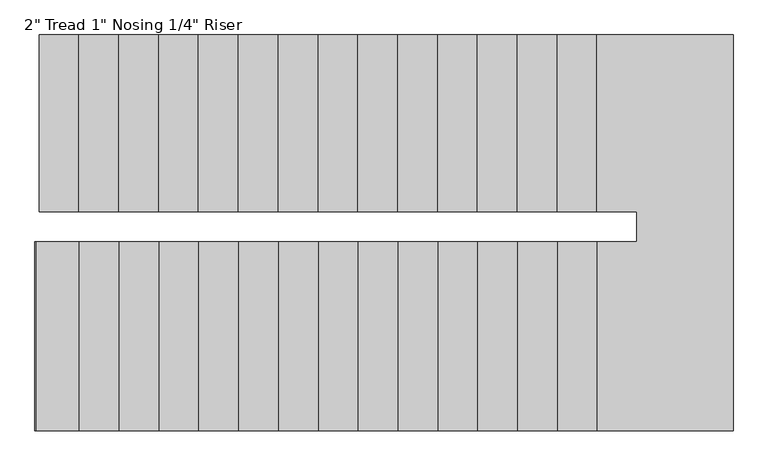
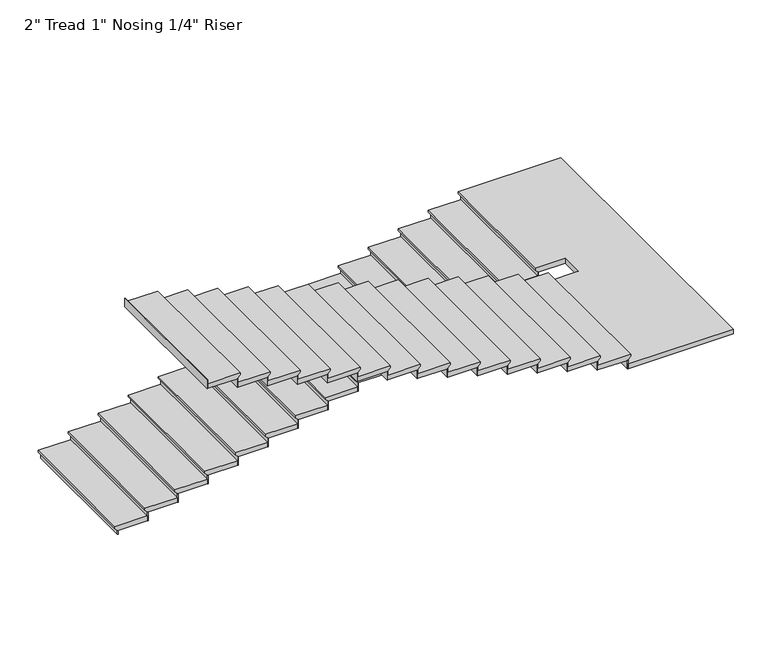
"""IFC4 building model written with IfcOpenShell, lengths in millimetres: stair flight geometry."""

from ifc_helpers import new_model, si_unit, origin, place, context, project, spatial, faceted_brep, source, transform, mapped, element, save


def stair_flight_aa8d9d08(model_context):
    return source(origin(), model_context, "Body", "Brep", [
        faceted_brep([(-5254.0891351, 11154.2082924, 9216.39), (-5254.0891351, 11154.2082924, 9235.44), (-5254.0891351, 12506.0715905, 9235.44), (-5254.0891351, 12506.0715905, 9216.39), (-5228.6891351, 11154.2082924, 9190.99), (-5228.6891351, 12506.0715905, 9190.99), (-4923.8891351, 11154.2082924, 9235.44), (-4923.8891351, 12506.0715905, 9235.44), (-5228.6891351, 12506.0715905, 9184.64), (-4923.8891351, 12506.0715905, 9184.64), (-4923.8891351, 11154.2082924, 9184.64), (-5228.6891351, 11154.2082924, 9184.64)], [[[0, 1, 2, 3]], [[4, 0, 3, 5]], [[2, 1, 6, 7]], [[8, 9, 10, 11]], [[2, 7, 9, 8, 5, 3]], [[8, 11, 4, 5]], [[6, 1, 0, 4, 11, 10]], [[7, 6, 10, 9]]]),
        faceted_brep([(-5228.6891351, 11154.2082924, 9184.64), (-5228.6891351, 11154.2082924, 9144.0), (-5222.3391351, 11154.2082924, 9144.0), (-5222.3391351, 11154.2082924, 9184.64), (-5228.6891351, 12506.0715905, 9184.64), (-5222.3391351, 12506.0715905, 9184.64), (-5222.3391351, 12506.0715905, 9144.0), (-5228.6891351, 12506.0715905, 9144.0)], [[[0, 1, 2, 3]], [[4, 5, 6, 7]], [[1, 0, 4, 7]], [[2, 1, 7, 6]], [[3, 2, 6, 5]], [[0, 3, 5, 4]]]),
        faceted_brep([(-4923.8891351, 11154.2082924, 9276.08), (-4923.8891351, 11154.2082924, 9184.64), (-4917.5391351, 11154.2082924, 9184.64), (-4917.5391351, 11154.2082924, 9276.08), (-4923.8891351, 12506.0715905, 9276.08), (-4917.5391351, 12506.0715905, 9276.08), (-4917.5391351, 12506.0715905, 9184.64), (-4923.8891351, 12506.0715905, 9184.64)], [[[0, 1, 2, 3]], [[4, 5, 6, 7]], [[1, 0, 4, 7]], [[2, 1, 7, 6]], [[3, 2, 6, 5]], [[0, 3, 5, 4]]]),
        faceted_brep([(-4949.2891351, 12506.0715905, 9326.88), (-4949.2891351, 11154.2082924, 9326.88), (-4619.0891351, 11154.2082924, 9326.88), (-4619.0891351, 12506.0715905, 9326.88), (-4923.8891351, 12506.0715905, 9276.08), (-4619.0891351, 12506.0715905, 9276.08), (-4619.0891351, 11154.2082924, 9276.08), (-4923.8891351, 11154.2082924, 9276.08), (-4923.8891351, 12506.0715905, 9282.43), (-4949.2891351, 12506.0715905, 9307.83), (-4923.8891351, 11154.2082924, 9282.43), (-4949.2891351, 11154.2082924, 9307.83)], [[[0, 1, 2, 3]], [[4, 5, 6, 7]], [[0, 3, 5, 4, 8, 9]], [[4, 7, 10, 8]], [[2, 1, 11, 10, 7, 6]], [[3, 2, 6, 5]], [[11, 1, 0, 9]], [[10, 11, 9, 8]]]),
        faceted_brep([(-4619.0891351, 11154.2082924, 9367.52), (-4619.0891351, 11154.2082924, 9276.08), (-4612.7391351, 11154.2082924, 9276.08), (-4612.7391351, 11154.2082924, 9367.52), (-4619.0891351, 12506.0715905, 9367.52), (-4612.7391351, 12506.0715905, 9367.52), (-4612.7391351, 12506.0715905, 9276.08), (-4619.0891351, 12506.0715905, 9276.08)], [[[0, 1, 2, 3]], [[4, 5, 6, 7]], [[1, 0, 4, 7]], [[2, 1, 7, 6]], [[3, 2, 6, 5]], [[0, 3, 5, 4]]]),
        faceted_brep([(-4644.4891351, 12506.0715905, 9418.32), (-4644.4891351, 11154.2082924, 9418.32), (-4314.2891351, 11154.2082924, 9418.32), (-4314.2891351, 12506.0715905, 9418.32), (-4619.0891351, 12506.0715905, 9367.52), (-4314.2891351, 12506.0715905, 9367.52), (-4314.2891351, 11154.2082924, 9367.52), (-4619.0891351, 11154.2082924, 9367.52), (-4619.0891351, 12506.0715905, 9373.87), (-4644.4891351, 12506.0715905, 9399.27), (-4619.0891351, 11154.2082924, 9373.87), (-4644.4891351, 11154.2082924, 9399.27)], [[[0, 1, 2, 3]], [[4, 5, 6, 7]], [[0, 3, 5, 4, 8, 9]], [[4, 7, 10, 8]], [[2, 1, 11, 10, 7, 6]], [[3, 2, 6, 5]], [[11, 1, 0, 9]], [[10, 11, 9, 8]]]),
        faceted_brep([(-4314.2891351, 11154.2082924, 9458.96), (-4314.2891351, 11154.2082924, 9367.52), (-4307.9391351, 11154.2082924, 9367.52), (-4307.9391351, 11154.2082924, 9458.96), (-4314.2891351, 12506.0715905, 9458.96), (-4307.9391351, 12506.0715905, 9458.96), (-4307.9391351, 12506.0715905, 9367.52), (-4314.2891351, 12506.0715905, 9367.52)], [[[0, 1, 2, 3]], [[4, 5, 6, 7]], [[1, 0, 4, 7]], [[2, 1, 7, 6]], [[3, 2, 6, 5]], [[0, 3, 5, 4]]]),
        faceted_brep([(-4339.6891351, 12506.0715905, 9509.76), (-4339.6891351, 11154.2082924, 9509.76), (-4009.4891351, 11154.2082924, 9509.76), (-4009.4891351, 12506.0715905, 9509.76), (-4314.2891351, 12506.0715905, 9458.96), (-4009.4891351, 12506.0715905, 9458.96), (-4009.4891351, 11154.2082924, 9458.96), (-4314.2891351, 11154.2082924, 9458.96), (-4314.2891351, 12506.0715905, 9465.31), (-4339.6891351, 12506.0715905, 9490.71), (-4314.2891351, 11154.2082924, 9465.31), (-4339.6891351, 11154.2082924, 9490.71)], [[[0, 1, 2, 3]], [[4, 5, 6, 7]], [[0, 3, 5, 4, 8, 9]], [[4, 7, 10, 8]], [[2, 1, 11, 10, 7, 6]], [[3, 2, 6, 5]], [[11, 1, 0, 9]], [[10, 11, 9, 8]]]),
        faceted_brep([(-4009.4891351, 11154.2082924, 9550.4), (-4009.4891351, 11154.2082924, 9458.96), (-4003.1391351, 11154.2082924, 9458.96), (-4003.1391351, 11154.2082924, 9550.4), (-4009.4891351, 12506.0715905, 9550.4), (-4003.1391351, 12506.0715905, 9550.4), (-4003.1391351, 12506.0715905, 9458.96), (-4009.4891351, 12506.0715905, 9458.96)], [[[0, 1, 2, 3]], [[4, 5, 6, 7]], [[1, 0, 4, 7]], [[2, 1, 7, 6]], [[3, 2, 6, 5]], [[0, 3, 5, 4]]]),
        faceted_brep([(-4034.8891351, 12506.0715905, 9601.2), (-4034.8891351, 11154.2082924, 9601.2), (-3704.6891351, 11154.2082924, 9601.2), (-3704.6891351, 12506.0715905, 9601.2), (-4009.4891351, 12506.0715905, 9550.4), (-3704.6891351, 12506.0715905, 9550.4), (-3704.6891351, 11154.2082924, 9550.4), (-4009.4891351, 11154.2082924, 9550.4), (-4009.4891351, 12506.0715905, 9556.75), (-4034.8891351, 12506.0715905, 9582.15), (-4009.4891351, 11154.2082924, 9556.75), (-4034.8891351, 11154.2082924, 9582.15)], [[[0, 1, 2, 3]], [[4, 5, 6, 7]], [[0, 3, 5, 4, 8, 9]], [[4, 7, 10, 8]], [[2, 1, 11, 10, 7, 6]], [[3, 2, 6, 5]], [[11, 1, 0, 9]], [[10, 11, 9, 8]]]),
        faceted_brep([(-3704.6891351, 11154.2082924, 9641.84), (-3704.6891351, 11154.2082924, 9550.4), (-3698.3391351, 11154.2082924, 9550.4), (-3698.3391351, 11154.2082924, 9641.84), (-3704.6891351, 12506.0715905, 9641.84), (-3698.3391351, 12506.0715905, 9641.84), (-3698.3391351, 12506.0715905, 9550.4), (-3704.6891351, 12506.0715905, 9550.4)], [[[0, 1, 2, 3]], [[4, 5, 6, 7]], [[1, 0, 4, 7]], [[2, 1, 7, 6]], [[3, 2, 6, 5]], [[0, 3, 5, 4]]]),
        faceted_brep([(-3730.0891351, 12506.0715905, 9692.64), (-3730.0891351, 11154.2082924, 9692.64), (-3399.8891351, 11154.2082924, 9692.64), (-3399.8891351, 12506.0715905, 9692.64), (-3704.6891351, 12506.0715905, 9641.84), (-3399.8891351, 12506.0715905, 9641.84), (-3399.8891351, 11154.2082924, 9641.84), (-3704.6891351, 11154.2082924, 9641.84), (-3704.6891351, 12506.0715905, 9648.19), (-3730.0891351, 12506.0715905, 9673.59), (-3704.6891351, 11154.2082924, 9648.19), (-3730.0891351, 11154.2082924, 9673.59)], [[[0, 1, 2, 3]], [[4, 5, 6, 7]], [[0, 3, 5, 4, 8, 9]], [[4, 7, 10, 8]], [[2, 1, 11, 10, 7, 6]], [[3, 2, 6, 5]], [[11, 1, 0, 9]], [[10, 11, 9, 8]]]),
        faceted_brep([(-3399.8891351, 11154.2082924, 9733.28), (-3399.8891351, 11154.2082924, 9641.84), (-3393.5391351, 11154.2082924, 9641.84), (-3393.5391351, 11154.2082924, 9733.28), (-3399.8891351, 12506.0715905, 9733.28), (-3393.5391351, 12506.0715905, 9733.28), (-3393.5391351, 12506.0715905, 9641.84), (-3399.8891351, 12506.0715905, 9641.84)], [[[0, 1, 2, 3]], [[4, 5, 6, 7]], [[1, 0, 4, 7]], [[2, 1, 7, 6]], [[3, 2, 6, 5]], [[0, 3, 5, 4]]]),
        faceted_brep([(-3425.2891351, 12506.0715905, 9784.08), (-3425.2891351, 11154.2082924, 9784.08), (-3095.0891351, 11154.2082924, 9784.08), (-3095.0891351, 12506.0715905, 9784.08), (-3399.8891351, 12506.0715905, 9733.28), (-3095.0891351, 12506.0715905, 9733.28), (-3095.0891351, 11154.2082924, 9733.28), (-3399.8891351, 11154.2082924, 9733.28), (-3399.8891351, 12506.0715905, 9739.63), (-3425.2891351, 12506.0715905, 9765.03), (-3399.8891351, 11154.2082924, 9739.63), (-3425.2891351, 11154.2082924, 9765.03)], [[[0, 1, 2, 3]], [[4, 5, 6, 7]], [[0, 3, 5, 4, 8, 9]], [[4, 7, 10, 8]], [[2, 1, 11, 10, 7, 6]], [[3, 2, 6, 5]], [[11, 1, 0, 9]], [[10, 11, 9, 8]]]),
        faceted_brep([(-3095.0891351, 11154.2082924, 9824.72), (-3095.0891351, 11154.2082924, 9733.28), (-3088.7391351, 11154.2082924, 9733.28), (-3088.7391351, 11154.2082924, 9824.72), (-3095.0891351, 12506.0715905, 9824.72), (-3088.7391351, 12506.0715905, 9824.72), (-3088.7391351, 12506.0715905, 9733.28), (-3095.0891351, 12506.0715905, 9733.28)], [[[0, 1, 2, 3]], [[4, 5, 6, 7]], [[1, 0, 4, 7]], [[2, 1, 7, 6]], [[3, 2, 6, 5]], [[0, 3, 5, 4]]]),
        faceted_brep([(-3120.4891351, 12506.0715905, 9875.52), (-3120.4891351, 11154.2082924, 9875.52), (-2790.2891351, 11154.2082924, 9875.52), (-2790.2891351, 12506.0715905, 9875.52), (-3095.0891351, 12506.0715905, 9824.72), (-2790.2891351, 12506.0715905, 9824.72), (-2790.2891351, 11154.2082924, 9824.72), (-3095.0891351, 11154.2082924, 9824.72), (-3095.0891351, 12506.0715905, 9831.07), (-3120.4891351, 12506.0715905, 9856.47), (-3095.0891351, 11154.2082924, 9831.07), (-3120.4891351, 11154.2082924, 9856.47)], [[[0, 1, 2, 3]], [[4, 5, 6, 7]], [[0, 3, 5, 4, 8, 9]], [[4, 7, 10, 8]], [[2, 1, 11, 10, 7, 6]], [[3, 2, 6, 5]], [[11, 1, 0, 9]], [[10, 11, 9, 8]]]),
        faceted_brep([(-2790.2891351, 11154.2082924, 9916.16), (-2790.2891351, 11154.2082924, 9824.72), (-2783.9391351, 11154.2082924, 9824.72), (-2783.9391351, 11154.2082924, 9916.16), (-2790.2891351, 12506.0715905, 9916.16), (-2783.9391351, 12506.0715905, 9916.16), (-2783.9391351, 12506.0715905, 9824.72), (-2790.2891351, 12506.0715905, 9824.72)], [[[0, 1, 2, 3]], [[4, 5, 6, 7]], [[1, 0, 4, 7]], [[2, 1, 7, 6]], [[3, 2, 6, 5]], [[0, 3, 5, 4]]]),
        faceted_brep([(-2815.6891351, 12506.0715905, 9966.96), (-2815.6891351, 11154.2082924, 9966.96), (-2485.4891351, 11154.2082924, 9966.96), (-2485.4891351, 12506.0715905, 9966.96), (-2790.2891351, 12506.0715905, 9916.16), (-2485.4891351, 12506.0715905, 9916.16), (-2485.4891351, 11154.2082924, 9916.16), (-2790.2891351, 11154.2082924, 9916.16), (-2790.2891351, 12506.0715905, 9922.51), (-2815.6891351, 12506.0715905, 9947.91), (-2790.2891351, 11154.2082924, 9922.51), (-2815.6891351, 11154.2082924, 9947.91)], [[[0, 1, 2, 3]], [[4, 5, 6, 7]], [[0, 3, 5, 4, 8, 9]], [[4, 7, 10, 8]], [[2, 1, 11, 10, 7, 6]], [[3, 2, 6, 5]], [[11, 1, 0, 9]], [[10, 11, 9, 8]]]),
        faceted_brep([(-2485.4891351, 11154.2082924, 10007.6), (-2485.4891351, 11154.2082924, 9916.16), (-2479.1391351, 11154.2082924, 9916.16), (-2479.1391351, 11154.2082924, 10007.6), (-2485.4891351, 12506.0715905, 10007.6), (-2479.1391351, 12506.0715905, 10007.6), (-2479.1391351, 12506.0715905, 9916.16), (-2485.4891351, 12506.0715905, 9916.16)], [[[0, 1, 2, 3]], [[4, 5, 6, 7]], [[1, 0, 4, 7]], [[2, 1, 7, 6]], [[3, 2, 6, 5]], [[0, 3, 5, 4]]]),
        faceted_brep([(-2510.8891351, 12506.0715905, 10058.4), (-2510.8891351, 11154.2082924, 10058.4), (-2180.6891351, 11154.2082924, 10058.4), (-2180.6891351, 12506.0715905, 10058.4), (-2485.4891351, 12506.0715905, 10007.6), (-2180.6891351, 12506.0715905, 10007.6), (-2180.6891351, 11154.2082924, 10007.6), (-2485.4891351, 11154.2082924, 10007.6), (-2485.4891351, 12506.0715905, 10013.95), (-2510.8891351, 12506.0715905, 10039.35), (-2485.4891351, 11154.2082924, 10013.95), (-2510.8891351, 11154.2082924, 10039.35)], [[[0, 1, 2, 3]], [[4, 5, 6, 7]], [[0, 3, 5, 4, 8, 9]], [[4, 7, 10, 8]], [[2, 1, 11, 10, 7, 6]], [[3, 2, 6, 5]], [[11, 1, 0, 9]], [[10, 11, 9, 8]]]),
        faceted_brep([(-2180.6891351, 11154.2082924, 10099.04), (-2180.6891351, 11154.2082924, 10007.6), (-2174.3391351, 11154.2082924, 10007.6), (-2174.3391351, 11154.2082924, 10099.04), (-2180.6891351, 12506.0715905, 10099.04), (-2174.3391351, 12506.0715905, 10099.04), (-2174.3391351, 12506.0715905, 10007.6), (-2180.6891351, 12506.0715905, 10007.6)], [[[0, 1, 2, 3]], [[4, 5, 6, 7]], [[1, 0, 4, 7]], [[2, 1, 7, 6]], [[3, 2, 6, 5]], [[0, 3, 5, 4]]]),
        faceted_brep([(-2206.0891351, 12506.0715905, 10149.84), (-2206.0891351, 11154.2082924, 10149.84), (-1875.8891351, 11154.2082924, 10149.84), (-1875.8891351, 12506.0715905, 10149.84), (-2180.6891351, 12506.0715905, 10099.04), (-1875.8891351, 12506.0715905, 10099.04), (-1875.8891351, 11154.2082924, 10099.04), (-2180.6891351, 11154.2082924, 10099.04), (-2180.6891351, 12506.0715905, 10105.39), (-2206.0891351, 12506.0715905, 10130.79), (-2180.6891351, 11154.2082924, 10105.39), (-2206.0891351, 11154.2082924, 10130.79)], [[[0, 1, 2, 3]], [[4, 5, 6, 7]], [[0, 3, 5, 4, 8, 9]], [[4, 7, 10, 8]], [[2, 1, 11, 10, 7, 6]], [[3, 2, 6, 5]], [[11, 1, 0, 9]], [[10, 11, 9, 8]]]),
        faceted_brep([(-1875.8891351, 11154.2082924, 10190.48), (-1875.8891351, 11154.2082924, 10099.04), (-1869.5391351, 11154.2082924, 10099.04), (-1869.5391351, 11154.2082924, 10190.48), (-1875.8891351, 12506.0715905, 10190.48), (-1869.5391351, 12506.0715905, 10190.48), (-1869.5391351, 12506.0715905, 10099.04), (-1875.8891351, 12506.0715905, 10099.04)], [[[0, 1, 2, 3]], [[4, 5, 6, 7]], [[1, 0, 4, 7]], [[2, 1, 7, 6]], [[3, 2, 6, 5]], [[0, 3, 5, 4]]]),
        faceted_brep([(-1901.2891351, 12506.0715905, 10241.28), (-1901.2891351, 11154.2082924, 10241.28), (-1571.0891351, 11154.2082924, 10241.28), (-1571.0891351, 12506.0715905, 10241.28), (-1875.8891351, 12506.0715905, 10190.48), (-1571.0891351, 12506.0715905, 10190.48), (-1571.0891351, 11154.2082924, 10190.48), (-1875.8891351, 11154.2082924, 10190.48), (-1875.8891351, 12506.0715905, 10196.83), (-1901.2891351, 12506.0715905, 10222.23), (-1875.8891351, 11154.2082924, 10196.83), (-1901.2891351, 11154.2082924, 10222.23)], [[[0, 1, 2, 3]], [[4, 5, 6, 7]], [[0, 3, 5, 4, 8, 9]], [[4, 7, 10, 8]], [[2, 1, 11, 10, 7, 6]], [[3, 2, 6, 5]], [[11, 1, 0, 9]], [[10, 11, 9, 8]]]),
        faceted_brep([(-1571.0891351, 11154.2082924, 10281.92), (-1571.0891351, 11154.2082924, 10190.48), (-1564.7391351, 11154.2082924, 10190.48), (-1564.7391351, 11154.2082924, 10281.92), (-1571.0891351, 12506.0715905, 10281.92), (-1564.7391351, 12506.0715905, 10281.92), (-1564.7391351, 12506.0715905, 10190.48), (-1571.0891351, 12506.0715905, 10190.48)], [[[0, 1, 2, 3]], [[4, 5, 6, 7]], [[1, 0, 4, 7]], [[2, 1, 7, 6]], [[3, 2, 6, 5]], [[0, 3, 5, 4]]]),
        faceted_brep([(-1596.4891351, 12506.0715905, 10332.72), (-1596.4891351, 11154.2082924, 10332.72), (-1266.2891351, 11154.2082924, 10332.72), (-1266.2891351, 12506.0715905, 10332.72), (-1571.0891351, 12506.0715905, 10281.92), (-1266.2891351, 12506.0715905, 10281.92), (-1266.2891351, 11154.2082924, 10281.92), (-1571.0891351, 11154.2082924, 10281.92), (-1571.0891351, 12506.0715905, 10288.27), (-1596.4891351, 12506.0715905, 10313.67), (-1571.0891351, 11154.2082924, 10288.27), (-1596.4891351, 11154.2082924, 10313.67)], [[[0, 1, 2, 3]], [[4, 5, 6, 7]], [[0, 3, 5, 4, 8, 9]], [[4, 7, 10, 8]], [[2, 1, 11, 10, 7, 6]], [[3, 2, 6, 5]], [[11, 1, 0, 9]], [[10, 11, 9, 8]]]),
        faceted_brep([(-1266.2891351, 11154.2082924, 10373.36), (-1266.2891351, 11154.2082924, 10281.92), (-1259.9391351, 11154.2082924, 10281.92), (-1259.9391351, 11154.2082924, 10373.36), (-1266.2891351, 12506.0715905, 10373.36), (-1259.9391351, 12506.0715905, 10373.36), (-1259.9391351, 12506.0715905, 10281.92), (-1266.2891351, 12506.0715905, 10281.92)], [[[0, 1, 2, 3]], [[4, 5, 6, 7]], [[1, 0, 4, 7]], [[2, 1, 7, 6]], [[3, 2, 6, 5]], [[0, 3, 5, 4]]]),
        faceted_brep([(-1291.6891351, 12506.0715905, 10424.16), (-1291.6891351, 11154.2082924, 10424.16), (-961.4891351, 11154.2082924, 10424.16), (-961.4891351, 12506.0715905, 10424.16), (-1266.2891351, 12506.0715905, 10373.36), (-961.4891351, 12506.0715905, 10373.36), (-961.4891351, 11154.2082924, 10373.36), (-1266.2891351, 11154.2082924, 10373.36), (-1266.2891351, 12506.0715905, 10379.71), (-1291.6891351, 12506.0715905, 10405.11), (-1266.2891351, 11154.2082924, 10379.71), (-1291.6891351, 11154.2082924, 10405.11)], [[[0, 1, 2, 3]], [[4, 5, 6, 7]], [[0, 3, 5, 4, 8, 9]], [[4, 7, 10, 8]], [[2, 1, 11, 10, 7, 6]], [[3, 2, 6, 5]], [[11, 1, 0, 9]], [[10, 11, 9, 8]]]),
        faceted_brep([(-961.4891351, 11154.2082924, 10464.8), (-961.4891351, 11154.2082924, 10373.36), (-955.1391351, 11154.2082924, 10373.36), (-955.1391351, 11154.2082924, 10464.8), (-961.4891351, 12506.0715905, 10464.8), (-955.1391351, 12506.0715905, 10464.8), (-955.1391351, 12506.0715905, 10373.36), (-961.4891351, 12506.0715905, 10373.36)], [[[0, 1, 2, 3]], [[4, 5, 6, 7]], [[1, 0, 4, 7]], [[2, 1, 7, 6]], [[3, 2, 6, 5]], [[0, 3, 5, 4]]]),
        faceted_brep([(-1012.2891351, 9478.4949943, 10515.6), (54.5108649, 9478.4949943, 10515.6), (54.5108649, 12506.0715905, 10515.6), (-986.8891351, 12506.0715905, 10515.6), (-986.8891351, 11154.2082924, 10515.6), (-682.0891351, 11154.2082924, 10515.6), (-682.0891351, 10925.6082924, 10515.6), (-1012.2891351, 10925.6082924, 10515.6), (54.5108649, 9478.4949943, 10464.8), (-1012.2891351, 9478.4949943, 10464.8), (-1012.2891351, 10925.6082924, 10464.8), (-682.0891351, 10925.6082924, 10464.8), (-682.0891351, 11154.2082924, 10464.8), (-961.4891351, 11154.2082924, 10464.8), (-961.4891351, 12506.0715905, 10464.8), (54.5108649, 12506.0715905, 10464.8), (-961.4891351, 12506.0715905, 10471.15), (-986.8891351, 12506.0715905, 10496.55), (-961.4891351, 11154.2082924, 10471.15), (-986.8891351, 11154.2082924, 10496.55)], [[[0, 1, 2, 3, 4, 5, 6, 7]], [[8, 9, 10, 11, 12, 13, 14, 15]], [[1, 0, 9, 8]], [[2, 1, 8, 15]], [[3, 2, 15, 14, 16, 17]], [[14, 13, 18, 16]], [[5, 4, 19, 18, 13, 12]], [[6, 5, 12, 11]], [[7, 6, 11, 10]], [[0, 7, 10, 9]], [[19, 4, 3, 17]], [[18, 19, 17, 16]]]),
        faceted_brep([(-1012.2891351, 10925.6082924, 10556.24), (-1012.2891351, 10925.6082924, 10464.8), (-1018.6391351, 10925.6082924, 10464.8), (-1018.6391351, 10925.6082924, 10556.24), (-1012.2891351, 9478.4949943, 10556.24), (-1018.6391351, 9478.4949943, 10556.24), (-1018.6391351, 9478.4949943, 10464.8), (-1012.2891351, 9478.4949943, 10464.8)], [[[0, 1, 2, 3]], [[4, 5, 6, 7]], [[1, 0, 4, 7]], [[2, 1, 7, 6]], [[3, 2, 6, 5]], [[0, 3, 5, 4]]]),
        faceted_brep([(-986.8891351, 9478.4949943, 10607.04), (-986.8891351, 10925.6082924, 10607.04), (-1317.0891351, 10925.6082924, 10607.04), (-1317.0891351, 9478.4949943, 10607.04), (-1012.2891351, 9478.4949943, 10556.24), (-1317.0891351, 9478.4949943, 10556.24), (-1317.0891351, 10925.6082924, 10556.24), (-1012.2891351, 10925.6082924, 10556.24), (-1012.2891351, 9478.4949943, 10562.59), (-986.8891351, 9478.4949943, 10587.99), (-1012.2891351, 10925.6082924, 10562.59), (-986.8891351, 10925.6082924, 10587.99)], [[[0, 1, 2, 3]], [[4, 5, 6, 7]], [[0, 3, 5, 4, 8, 9]], [[4, 7, 10, 8]], [[2, 1, 11, 10, 7, 6]], [[3, 2, 6, 5]], [[11, 1, 0, 9]], [[10, 11, 9, 8]]]),
        faceted_brep([(-1317.0891351, 10925.6082924, 10647.68), (-1317.0891351, 10925.6082924, 10556.24), (-1323.4391351, 10925.6082924, 10556.24), (-1323.4391351, 10925.6082924, 10647.68), (-1317.0891351, 9478.4949943, 10647.68), (-1323.4391351, 9478.4949943, 10647.68), (-1323.4391351, 9478.4949943, 10556.24), (-1317.0891351, 9478.4949943, 10556.24)], [[[0, 1, 2, 3]], [[4, 5, 6, 7]], [[1, 0, 4, 7]], [[2, 1, 7, 6]], [[3, 2, 6, 5]], [[0, 3, 5, 4]]]),
        faceted_brep([(-1291.6891351, 9478.4949943, 10698.48), (-1291.6891351, 10925.6082924, 10698.48), (-1621.8891351, 10925.6082924, 10698.48), (-1621.8891351, 9478.4949943, 10698.48), (-1317.0891351, 9478.4949943, 10647.68), (-1621.8891351, 9478.4949943, 10647.68), (-1621.8891351, 10925.6082924, 10647.68), (-1317.0891351, 10925.6082924, 10647.68), (-1317.0891351, 9478.4949943, 10654.03), (-1291.6891351, 9478.4949943, 10679.43), (-1317.0891351, 10925.6082924, 10654.03), (-1291.6891351, 10925.6082924, 10679.43)], [[[0, 1, 2, 3]], [[4, 5, 6, 7]], [[0, 3, 5, 4, 8, 9]], [[4, 7, 10, 8]], [[2, 1, 11, 10, 7, 6]], [[3, 2, 6, 5]], [[11, 1, 0, 9]], [[10, 11, 9, 8]]]),
        faceted_brep([(-1621.8891351, 10925.6082924, 10739.12), (-1621.8891351, 10925.6082924, 10647.68), (-1628.2391351, 10925.6082924, 10647.68), (-1628.2391351, 10925.6082924, 10739.12), (-1621.8891351, 9478.4949943, 10739.12), (-1628.2391351, 9478.4949943, 10739.12), (-1628.2391351, 9478.4949943, 10647.68), (-1621.8891351, 9478.4949943, 10647.68)], [[[0, 1, 2, 3]], [[4, 5, 6, 7]], [[1, 0, 4, 7]], [[2, 1, 7, 6]], [[3, 2, 6, 5]], [[0, 3, 5, 4]]]),
        faceted_brep([(-1596.4891351, 9478.4949943, 10789.92), (-1596.4891351, 10925.6082924, 10789.92), (-1926.6891351, 10925.6082924, 10789.92), (-1926.6891351, 9478.4949943, 10789.92), (-1621.8891351, 9478.4949943, 10739.12), (-1926.6891351, 9478.4949943, 10739.12), (-1926.6891351, 10925.6082924, 10739.12), (-1621.8891351, 10925.6082924, 10739.12), (-1621.8891351, 9478.4949943, 10745.47), (-1596.4891351, 9478.4949943, 10770.87), (-1621.8891351, 10925.6082924, 10745.47), (-1596.4891351, 10925.6082924, 10770.87)], [[[0, 1, 2, 3]], [[4, 5, 6, 7]], [[0, 3, 5, 4, 8, 9]], [[4, 7, 10, 8]], [[2, 1, 11, 10, 7, 6]], [[3, 2, 6, 5]], [[11, 1, 0, 9]], [[10, 11, 9, 8]]]),
        faceted_brep([(-1926.6891351, 10925.6082924, 10830.56), (-1926.6891351, 10925.6082924, 10739.12), (-1933.0391351, 10925.6082924, 10739.12), (-1933.0391351, 10925.6082924, 10830.56), (-1926.6891351, 9478.4949943, 10830.56), (-1933.0391351, 9478.4949943, 10830.56), (-1933.0391351, 9478.4949943, 10739.12), (-1926.6891351, 9478.4949943, 10739.12)], [[[0, 1, 2, 3]], [[4, 5, 6, 7]], [[1, 0, 4, 7]], [[2, 1, 7, 6]], [[3, 2, 6, 5]], [[0, 3, 5, 4]]]),
        faceted_brep([(-1901.2891351, 9478.4949943, 10881.36), (-1901.2891351, 10925.6082924, 10881.36), (-2231.4891351, 10925.6082924, 10881.36), (-2231.4891351, 9478.4949943, 10881.36), (-1926.6891351, 9478.4949943, 10830.56), (-2231.4891351, 9478.4949943, 10830.56), (-2231.4891351, 10925.6082924, 10830.56), (-1926.6891351, 10925.6082924, 10830.56), (-1926.6891351, 9478.4949943, 10836.91), (-1901.2891351, 9478.4949943, 10862.31), (-1926.6891351, 10925.6082924, 10836.91), (-1901.2891351, 10925.6082924, 10862.31)], [[[0, 1, 2, 3]], [[4, 5, 6, 7]], [[0, 3, 5, 4, 8, 9]], [[4, 7, 10, 8]], [[2, 1, 11, 10, 7, 6]], [[3, 2, 6, 5]], [[11, 1, 0, 9]], [[10, 11, 9, 8]]]),
        faceted_brep([(-2231.4891351, 10925.6082924, 10922.0), (-2231.4891351, 10925.6082924, 10830.56), (-2237.8391351, 10925.6082924, 10830.56), (-2237.8391351, 10925.6082924, 10922.0), (-2231.4891351, 9478.4949943, 10922.0), (-2237.8391351, 9478.4949943, 10922.0), (-2237.8391351, 9478.4949943, 10830.56), (-2231.4891351, 9478.4949943, 10830.56)], [[[0, 1, 2, 3]], [[4, 5, 6, 7]], [[1, 0, 4, 7]], [[2, 1, 7, 6]], [[3, 2, 6, 5]], [[0, 3, 5, 4]]]),
        faceted_brep([(-2206.0891351, 9478.4949943, 10972.8), (-2206.0891351, 10925.6082924, 10972.8), (-2536.2891351, 10925.6082924, 10972.8), (-2536.2891351, 9478.4949943, 10972.8), (-2231.4891351, 9478.4949943, 10922.0), (-2536.2891351, 9478.4949943, 10922.0), (-2536.2891351, 10925.6082924, 10922.0), (-2231.4891351, 10925.6082924, 10922.0), (-2231.4891351, 9478.4949943, 10928.35), (-2206.0891351, 9478.4949943, 10953.75), (-2231.4891351, 10925.6082924, 10928.35), (-2206.0891351, 10925.6082924, 10953.75)], [[[0, 1, 2, 3]], [[4, 5, 6, 7]], [[0, 3, 5, 4, 8, 9]], [[4, 7, 10, 8]], [[2, 1, 11, 10, 7, 6]], [[3, 2, 6, 5]], [[11, 1, 0, 9]], [[10, 11, 9, 8]]]),
        faceted_brep([(-2536.2891351, 10925.6082924, 11013.44), (-2536.2891351, 10925.6082924, 10922.0), (-2542.6391351, 10925.6082924, 10922.0), (-2542.6391351, 10925.6082924, 11013.44), (-2536.2891351, 9478.4949943, 11013.44), (-2542.6391351, 9478.4949943, 11013.44), (-2542.6391351, 9478.4949943, 10922.0), (-2536.2891351, 9478.4949943, 10922.0)], [[[0, 1, 2, 3]], [[4, 5, 6, 7]], [[1, 0, 4, 7]], [[2, 1, 7, 6]], [[3, 2, 6, 5]], [[0, 3, 5, 4]]]),
        faceted_brep([(-2510.8891351, 9478.4949943, 11064.24), (-2510.8891351, 10925.6082924, 11064.24), (-2841.0891351, 10925.6082924, 11064.24), (-2841.0891351, 9478.4949943, 11064.24), (-2536.2891351, 9478.4949943, 11013.44), (-2841.0891351, 9478.4949943, 11013.44), (-2841.0891351, 10925.6082924, 11013.44), (-2536.2891351, 10925.6082924, 11013.44), (-2536.2891351, 9478.4949943, 11019.79), (-2510.8891351, 9478.4949943, 11045.19), (-2536.2891351, 10925.6082924, 11019.79), (-2510.8891351, 10925.6082924, 11045.19)], [[[0, 1, 2, 3]], [[4, 5, 6, 7]], [[0, 3, 5, 4, 8, 9]], [[4, 7, 10, 8]], [[2, 1, 11, 10, 7, 6]], [[3, 2, 6, 5]], [[11, 1, 0, 9]], [[10, 11, 9, 8]]]),
        faceted_brep([(-2841.0891351, 10925.6082924, 11104.88), (-2841.0891351, 10925.6082924, 11013.44), (-2847.4391351, 10925.6082924, 11013.44), (-2847.4391351, 10925.6082924, 11104.88), (-2841.0891351, 9478.4949943, 11104.88), (-2847.4391351, 9478.4949943, 11104.88), (-2847.4391351, 9478.4949943, 11013.44), (-2841.0891351, 9478.4949943, 11013.44)], [[[0, 1, 2, 3]], [[4, 5, 6, 7]], [[1, 0, 4, 7]], [[2, 1, 7, 6]], [[3, 2, 6, 5]], [[0, 3, 5, 4]]]),
        faceted_brep([(-2815.6891351, 9478.4949943, 11155.68), (-2815.6891351, 10925.6082924, 11155.68), (-3145.8891351, 10925.6082924, 11155.68), (-3145.8891351, 9478.4949943, 11155.68), (-2841.0891351, 9478.4949943, 11104.88), (-3145.8891351, 9478.4949943, 11104.88), (-3145.8891351, 10925.6082924, 11104.88), (-2841.0891351, 10925.6082924, 11104.88), (-2841.0891351, 9478.4949943, 11111.23), (-2815.6891351, 9478.4949943, 11136.63), (-2841.0891351, 10925.6082924, 11111.23), (-2815.6891351, 10925.6082924, 11136.63)], [[[0, 1, 2, 3]], [[4, 5, 6, 7]], [[0, 3, 5, 4, 8, 9]], [[4, 7, 10, 8]], [[2, 1, 11, 10, 7, 6]], [[3, 2, 6, 5]], [[11, 1, 0, 9]], [[10, 11, 9, 8]]]),
        faceted_brep([(-3145.8891351, 10925.6082924, 11196.32), (-3145.8891351, 10925.6082924, 11104.88), (-3152.2391351, 10925.6082924, 11104.88), (-3152.2391351, 10925.6082924, 11196.32), (-3145.8891351, 9478.4949943, 11196.32), (-3152.2391351, 9478.4949943, 11196.32), (-3152.2391351, 9478.4949943, 11104.88), (-3145.8891351, 9478.4949943, 11104.88)], [[[0, 1, 2, 3]], [[4, 5, 6, 7]], [[1, 0, 4, 7]], [[2, 1, 7, 6]], [[3, 2, 6, 5]], [[0, 3, 5, 4]]]),
        faceted_brep([(-3120.4891351, 9478.4949943, 11247.12), (-3120.4891351, 10925.6082924, 11247.12), (-3450.6891351, 10925.6082924, 11247.12), (-3450.6891351, 9478.4949943, 11247.12), (-3145.8891351, 9478.4949943, 11196.32), (-3450.6891351, 9478.4949943, 11196.32), (-3450.6891351, 10925.6082924, 11196.32), (-3145.8891351, 10925.6082924, 11196.32), (-3145.8891351, 9478.4949943, 11202.67), (-3120.4891351, 9478.4949943, 11228.07), (-3145.8891351, 10925.6082924, 11202.67), (-3120.4891351, 10925.6082924, 11228.07)], [[[0, 1, 2, 3]], [[4, 5, 6, 7]], [[0, 3, 5, 4, 8, 9]], [[4, 7, 10, 8]], [[2, 1, 11, 10, 7, 6]], [[3, 2, 6, 5]], [[11, 1, 0, 9]], [[10, 11, 9, 8]]]),
        faceted_brep([(-3450.6891351, 10925.6082924, 11287.76), (-3450.6891351, 10925.6082924, 11196.32), (-3457.0391351, 10925.6082924, 11196.32), (-3457.0391351, 10925.6082924, 11287.76), (-3450.6891351, 9478.4949943, 11287.76), (-3457.0391351, 9478.4949943, 11287.76), (-3457.0391351, 9478.4949943, 11196.32), (-3450.6891351, 9478.4949943, 11196.32)], [[[0, 1, 2, 3]], [[4, 5, 6, 7]], [[1, 0, 4, 7]], [[2, 1, 7, 6]], [[3, 2, 6, 5]], [[0, 3, 5, 4]]]),
        faceted_brep([(-3425.2891351, 9478.4949943, 11338.56), (-3425.2891351, 10925.6082924, 11338.56), (-3755.4891351, 10925.6082924, 11338.56), (-3755.4891351, 9478.4949943, 11338.56), (-3450.6891351, 9478.4949943, 11287.76), (-3755.4891351, 9478.4949943, 11287.76), (-3755.4891351, 10925.6082924, 11287.76), (-3450.6891351, 10925.6082924, 11287.76), (-3450.6891351, 9478.4949943, 11294.11), (-3425.2891351, 9478.4949943, 11319.51), (-3450.6891351, 10925.6082924, 11294.11), (-3425.2891351, 10925.6082924, 11319.51)], [[[0, 1, 2, 3]], [[4, 5, 6, 7]], [[0, 3, 5, 4, 8, 9]], [[4, 7, 10, 8]], [[2, 1, 11, 10, 7, 6]], [[3, 2, 6, 5]], [[11, 1, 0, 9]], [[10, 11, 9, 8]]]),
        faceted_brep([(-3755.4891351, 10925.6082924, 11379.2), (-3755.4891351, 10925.6082924, 11287.76), (-3761.8391351, 10925.6082924, 11287.76), (-3761.8391351, 10925.6082924, 11379.2), (-3755.4891351, 9478.4949943, 11379.2), (-3761.8391351, 9478.4949943, 11379.2), (-3761.8391351, 9478.4949943, 11287.76), (-3755.4891351, 9478.4949943, 11287.76)], [[[0, 1, 2, 3]], [[4, 5, 6, 7]], [[1, 0, 4, 7]], [[2, 1, 7, 6]], [[3, 2, 6, 5]], [[0, 3, 5, 4]]]),
        faceted_brep([(-3730.0891351, 9478.4949943, 11430.0), (-3730.0891351, 10925.6082924, 11430.0), (-4060.2891351, 10925.6082924, 11430.0), (-4060.2891351, 9478.4949943, 11430.0), (-3755.4891351, 9478.4949943, 11379.2), (-4060.2891351, 9478.4949943, 11379.2), (-4060.2891351, 10925.6082924, 11379.2), (-3755.4891351, 10925.6082924, 11379.2), (-3755.4891351, 9478.4949943, 11385.55), (-3730.0891351, 9478.4949943, 11410.95), (-3755.4891351, 10925.6082924, 11385.55), (-3730.0891351, 10925.6082924, 11410.95)], [[[0, 1, 2, 3]], [[4, 5, 6, 7]], [[0, 3, 5, 4, 8, 9]], [[4, 7, 10, 8]], [[2, 1, 11, 10, 7, 6]], [[3, 2, 6, 5]], [[11, 1, 0, 9]], [[10, 11, 9, 8]]]),
        faceted_brep([(-4060.2891351, 10925.6082924, 11470.64), (-4060.2891351, 10925.6082924, 11379.2), (-4066.6391351, 10925.6082924, 11379.2), (-4066.6391351, 10925.6082924, 11470.64), (-4060.2891351, 9478.4949943, 11470.64), (-4066.6391351, 9478.4949943, 11470.64), (-4066.6391351, 9478.4949943, 11379.2), (-4060.2891351, 9478.4949943, 11379.2)], [[[0, 1, 2, 3]], [[4, 5, 6, 7]], [[1, 0, 4, 7]], [[2, 1, 7, 6]], [[3, 2, 6, 5]], [[0, 3, 5, 4]]]),
        faceted_brep([(-4034.8891351, 9478.4949943, 11521.44), (-4034.8891351, 10925.6082924, 11521.44), (-4365.0891351, 10925.6082924, 11521.44), (-4365.0891351, 9478.4949943, 11521.44), (-4060.2891351, 9478.4949943, 11470.64), (-4365.0891351, 9478.4949943, 11470.64), (-4365.0891351, 10925.6082924, 11470.64), (-4060.2891351, 10925.6082924, 11470.64), (-4060.2891351, 9478.4949943, 11476.99), (-4034.8891351, 9478.4949943, 11502.39), (-4060.2891351, 10925.6082924, 11476.99), (-4034.8891351, 10925.6082924, 11502.39)], [[[0, 1, 2, 3]], [[4, 5, 6, 7]], [[0, 3, 5, 4, 8, 9]], [[4, 7, 10, 8]], [[2, 1, 11, 10, 7, 6]], [[3, 2, 6, 5]], [[11, 1, 0, 9]], [[10, 11, 9, 8]]]),
        faceted_brep([(-4365.0891351, 10925.6082924, 11562.08), (-4365.0891351, 10925.6082924, 11470.64), (-4371.4391351, 10925.6082924, 11470.64), (-4371.4391351, 10925.6082924, 11562.08), (-4365.0891351, 9478.4949943, 11562.08), (-4371.4391351, 9478.4949943, 11562.08), (-4371.4391351, 9478.4949943, 11470.64), (-4365.0891351, 9478.4949943, 11470.64)], [[[0, 1, 2, 3]], [[4, 5, 6, 7]], [[1, 0, 4, 7]], [[2, 1, 7, 6]], [[3, 2, 6, 5]], [[0, 3, 5, 4]]]),
        faceted_brep([(-4339.6891351, 9478.4949943, 11612.88), (-4339.6891351, 10925.6082924, 11612.88), (-4669.8891351, 10925.6082924, 11612.88), (-4669.8891351, 9478.4949943, 11612.88), (-4365.0891351, 9478.4949943, 11562.08), (-4669.8891351, 9478.4949943, 11562.08), (-4669.8891351, 10925.6082924, 11562.08), (-4365.0891351, 10925.6082924, 11562.08), (-4365.0891351, 9478.4949943, 11568.43), (-4339.6891351, 9478.4949943, 11593.83), (-4365.0891351, 10925.6082924, 11568.43), (-4339.6891351, 10925.6082924, 11593.83)], [[[0, 1, 2, 3]], [[4, 5, 6, 7]], [[0, 3, 5, 4, 8, 9]], [[4, 7, 10, 8]], [[2, 1, 11, 10, 7, 6]], [[3, 2, 6, 5]], [[11, 1, 0, 9]], [[10, 11, 9, 8]]]),
        faceted_brep([(-4669.8891351, 10925.6082924, 11653.52), (-4669.8891351, 10925.6082924, 11562.08), (-4676.2391351, 10925.6082924, 11562.08), (-4676.2391351, 10925.6082924, 11653.52), (-4669.8891351, 9478.4949943, 11653.52), (-4676.2391351, 9478.4949943, 11653.52), (-4676.2391351, 9478.4949943, 11562.08), (-4669.8891351, 9478.4949943, 11562.08)], [[[0, 1, 2, 3]], [[4, 5, 6, 7]], [[1, 0, 4, 7]], [[2, 1, 7, 6]], [[3, 2, 6, 5]], [[0, 3, 5, 4]]]),
        faceted_brep([(-4644.4891351, 9478.4949943, 11704.32), (-4644.4891351, 10925.6082924, 11704.32), (-4974.6891351, 10925.6082924, 11704.32), (-4974.6891351, 9478.4949943, 11704.32), (-4669.8891351, 9478.4949943, 11653.52), (-4974.6891351, 9478.4949943, 11653.52), (-4974.6891351, 10925.6082924, 11653.52), (-4669.8891351, 10925.6082924, 11653.52), (-4669.8891351, 9478.4949943, 11659.87), (-4644.4891351, 9478.4949943, 11685.27), (-4669.8891351, 10925.6082924, 11659.87), (-4644.4891351, 10925.6082924, 11685.27)], [[[0, 1, 2, 3]], [[4, 5, 6, 7]], [[0, 3, 5, 4, 8, 9]], [[4, 7, 10, 8]], [[2, 1, 11, 10, 7, 6]], [[3, 2, 6, 5]], [[11, 1, 0, 9]], [[10, 11, 9, 8]]]),
        faceted_brep([(-4974.6891351, 10925.6082924, 11744.96), (-4974.6891351, 10925.6082924, 11653.52), (-4981.0391351, 10925.6082924, 11653.52), (-4981.0391351, 10925.6082924, 11744.96), (-4974.6891351, 9478.4949943, 11744.96), (-4981.0391351, 9478.4949943, 11744.96), (-4981.0391351, 9478.4949943, 11653.52), (-4974.6891351, 9478.4949943, 11653.52)], [[[0, 1, 2, 3]], [[4, 5, 6, 7]], [[1, 0, 4, 7]], [[2, 1, 7, 6]], [[3, 2, 6, 5]], [[0, 3, 5, 4]]]),
        faceted_brep([(-5279.4891351, 10925.6082924, 11836.4), (-5279.4891351, 10925.6082924, 11744.96), (-5285.8391351, 10925.6082924, 11744.96), (-5285.8391351, 10925.6082924, 11836.4), (-5279.4891351, 9478.4949943, 11836.4), (-5285.8391351, 9478.4949943, 11836.4), (-5285.8391351, 9478.4949943, 11744.96), (-5279.4891351, 9478.4949943, 11744.96)], [[[0, 1, 2, 3]], [[4, 5, 6, 7]], [[1, 0, 4, 7]], [[2, 1, 7, 6]], [[3, 2, 6, 5]], [[0, 3, 5, 4]]]),
        faceted_brep([(-4949.2891351, 9478.4949943, 11795.76), (-4949.2891351, 10925.6082924, 11795.76), (-5279.4891351, 10925.6082924, 11795.76), (-5279.4891351, 9478.4949943, 11795.76), (-4974.6891351, 9478.4949943, 11744.96), (-5279.4891351, 9478.4949943, 11744.96), (-5279.4891351, 10925.6082924, 11744.96), (-4974.6891351, 10925.6082924, 11744.96), (-4974.6891351, 9478.4949943, 11751.31), (-4949.2891351, 9478.4949943, 11776.71), (-4974.6891351, 10925.6082924, 11751.31), (-4949.2891351, 10925.6082924, 11776.71)], [[[0, 1, 2, 3]], [[4, 5, 6, 7]], [[0, 3, 5, 4, 8, 9]], [[4, 7, 10, 8]], [[2, 1, 11, 10, 7, 6]], [[3, 2, 6, 5]], [[11, 1, 0, 9]], [[10, 11, 9, 8]]]),
    ])


if __name__ == "__main__":
    model = new_model("IFC4")
    model_context = context("Model", 3, world=origin())
    ifc_project = project(units=[si_unit("LENGTHUNIT", "METRE", prefix="MILLI")], contexts=[model_context])
    site = spatial("IfcSite", under=ifc_project)
    building = spatial("IfcBuilding", under=site)
    placement = place(None, origin())
    stair_flight_shape = stair_flight_aa8d9d08(model_context)
    element("IfcStairFlight", 1, ObjectType="2\" Tread 1\" Nosing 1/4\" Riser", at=placement, inside=building, context=model_context, shape_type="MappedRepresentation", body=[
        mapped(stair_flight_shape, transform((0.0, 0.0, 0.0), x_axis=(1.0, 0.0, 0.0), y_axis=(0.0, 1.0, 0.0), z_axis=(0.0, 0.0, 1.0))),
    ])
    save(model, "model.ifc")
